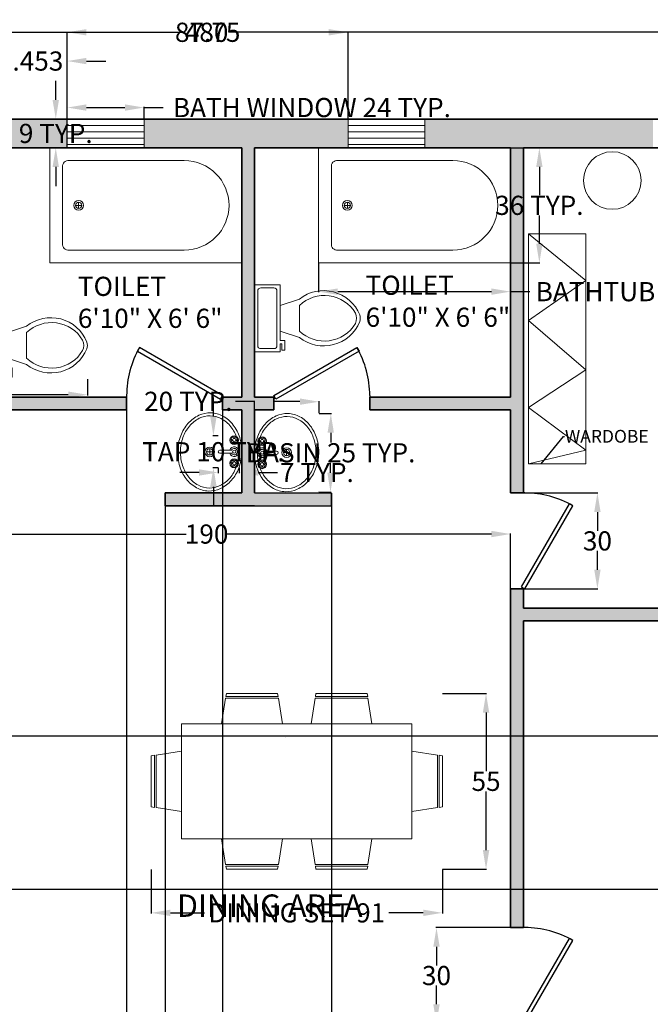
# Model space of a CAD drawing. Units: inches. Extents: x -16 to 578, y -553 to 49.
# Tile 4 of 5: x 205 to 402, y -259 to 49. Entities that reach past the tile are written whole.
import ezdxf
from ezdxf import colors
from ezdxf.entities.mleader import LeaderData, LeaderLine
from ezdxf.math import Vec2, Vec3

# ---------------------------------------------------------------- set-up
doc = ezdxf.new("R2010")
doc.units = ezdxf.units.IN
doc.header["$MEASUREMENT"] = 0
for name, color, linetype, lineweight in [('A-ANNO-DIMS', 2, 'Continuous', 18), ('A-ANNO-TEXT', 7, 'Continuous', 18), ('A-AREA-IDEN', 7, 'Continuous', 25), ('A-DOOR', 3, 'Continuous', 25), ('A-FLOR-CASE', 8, 'Continuous', 18), ('A-FLOR-FIXT', 9, 'Continuous', 18), ('A-FURN', 8, 'Continuous', 18), ('A-GLAZ', 4, 'Continuous', 18), ('A-WALL', 7, 'Continuous', 35)]:
    doc.layers.add(name, color=color, linetype=linetype, lineweight=lineweight)
doc.layers.add('A-WALL-PATT', color=251, linetype='Continuous', lineweight=13, true_color=0x636466)
doc.styles.get("Standard").update_dxf_attribs({"font": 'arial.ttf'})
doc.dimstyles.get("Standard").update_dxf_attribs({"dimtxt": 6, "dimasz": 6, "dimexe": 0.18, "dimexo": 0.0625, "dimgap": 0.09, "dimtad": 0, "dimtih": 1, "dimtoh": 1, "dimdec": 0, "dimzin": 0, "dimdsep": 46, "dimlunit": 4, "dimtxsty": 'Standard', "dimcen": 0.09, "dimadec": 0, "dimazin": 0, "dimtfac": 1, "dimtdec": 0, "dimtofl": 0, "dimtmove": 0, "dimatfit": 3, "dimfxl": 1, "dimtolj": 1, "dimtzin": 0, "dimarcsym": 0})

# ---------------------------------------------------------------- blocks, each defined once
blk = doc.blocks.new('*U4')
for p, q in [((0, 0), (0, -6)), ((-40, 0), (-40, -6))]:
    blk.add_line(p, q)
blk.add_lwpolyline([(0, 0), (-34.64, 20), (-35.52, 18.48), (-0.88, -1.52)], close=True)
blk.add_arc((0, 0), 40, 150, 180)
blk = doc.blocks.new('*U2')
for p, q in [((0, 0), (0, -6)), ((40, 0), (40, -6))]:
    blk.add_line(p, q)
blk.add_lwpolyline([(0, 0), (34.64, 20), (35.52, 18.48), (0.87, -1.52)], close=True)
blk.add_arc((0, 0), 40, 0, 30)
blk = doc.blocks.new('Toilet - top')
for p, q in [((9.5, -6), (9.5, -2)), ((-10, -8.5), (-8, -8.5)), ((-10, -9.5), (-10, -8.5)), ((-8, -8.5), (-8, -8)), ((-7, -8), (-7, -9.5)), ((-4, -8), (-6, -14)), ((4, -8), (6, -14)), ((-7, -9.5), (-10, -9.5)), ((4, -14), (-4, -14))]:
    blk.add_line(p, q)
for points in [[(-7, -8), (10.5, -8), (10.5, 0), (-10.5, 0), (-10.5, -8), (-8, -8)], [(-9.5, -2), (-9.5, -6)], [(8.5, -1), (-8.5, -1)], [(-8.5, -7), (8.5, -7)]]:
    blk.add_lwpolyline(points)
for centre, radius, start, end in [((-8.62, -1.88), 0.884, 81.8699, 188.1301), ((8.62, -1.88), 0.884, 351.8699, 98.1301), ((-8.62, -6.12), 0.884, 171.8699, 278.1301), ((8.62, -6.12), 0.884, 261.8699, 8.1301), ((3.52, -21.58), 12.17, 141.4691, 247.9714), ((4.2, -21.82), 11.33, 136.3677, 238.9468), ((-3.52, -21.58), 12.17, 292.0284, 38.5307), ((-4.2, -21.82), 11.33, 301.053, 43.6321), ((0, -27.88), 4, 245.7318, 294.2682), ((0, -29), 4, 254.8605, 285.1395)]:
    blk.add_arc(centre, radius, start, end)
blk = doc.blocks.new('Bath Tub - 26 x 60 in.')
for p, q in [((8, -18), (10, -18)), ((9, -17), (9, -19))]:
    blk.add_line(p, q)
blk.add_lwpolyline([(0, -36), (0, 0), (60, 0), (60, -36)], close=True)
for points in [[(4, -30), (4, -6)], [(6, -4), (42, -4)], [(42, -32), (6, -32)]]:
    blk.add_lwpolyline(points)
for radius in [1.5, 1]:
    blk.add_circle((9, -18), radius)
for centre, radius, start, end in [((5.75, -5.75), 1.77, 81.8699, 188.1301), ((42, -18), 14, 270, 90), ((5.75, -30.25), 1.77, 171.8699, 278.1301)]:
    blk.add_arc(centre, radius, start, end)
blk = doc.blocks.new('Sink - Oval top')
for p, q in [((-1, 0), (1, 0)), ((0, 1), (0, -1))]:
    blk.add_line(p, q)
for points in [[(-12.23, 0.39, 0.117634), (-11.46, -3.36, 0.104469), (-8.88, -6.8, 0.090016), (-5.08, -9.07, 0.08192), (-0.32, -10.02, 0.08192), (4.49, -9.38, 0.090016), (8.42, -7.36, 0.104469), (11.22, -4.09, 0.117634), (12.23, -0.39, 0.117634), (11.46, 3.36, 0.104469), (8.88, 6.8, 0.090016), (5.08, 9.07, 0.08192), (0.32, 10.02, 0.08192), (-4.49, 9.38, 0.090016), (-8.42, 7.36, 0.104469), (-11.22, 4.09, 0.117634)], [(-11.29, 0.16, 0.118622), (-10.52, -3.25, 0.104678), (-8.07, -6.36, 0.089562), (-4.54, -8.37, 0.081185), (-0.13, -9.15, 0.081185), (4.3, -8.49, 0.089562), (7.89, -6.58, 0.104678), (10.42, -3.55, 0.118622), (11.29, -0.16, 0.118622), (10.52, 3.25, 0.104678), (8.07, 6.36, 0.089562), (4.54, 8.37, 0.081185), (0.13, 9.15, 0.081185), (-4.3, 8.49, 0.089562), (-7.89, 6.58, 0.104678), (-10.42, 3.55, 0.118622)]]:
    blk.add_lwpolyline(points, format="xyb", close=True)
for radius in [1.5, 1]:
    blk.add_circle((0, 0), radius)
blk = doc.blocks.new('Faucet - Bathroom top')
for p, q in [((-4.107, 0.125), (-4.375, 0.125)), ((-3.75, 0.4788), (-3.75, 0.75)), ((-3.5, 0.482), (-3.5, 0.75)), ((-3.1461, 0.125), (-2.875, 0.125)), ((3.143, 0.125), (2.875, 0.125)), ((3.5, 0.4788), (3.5, 0.75)), ((3.75, 0.482), (3.75, 0.75)), ((4.1039, 0.125), (4.375, 0.125)), ((-4.1039, -0.125), (-4.375, -0.125)), ((-3.75, -0.4821), (-3.75, -0.75)), ((-3.5, -0.4789), (-3.5, -0.75)), ((-3.143, -0.125), (-2.875, -0.125)), ((-0.5, -0.8639), (-0.5, -4.5)), ((0.5, -4.5), (0.5, -0.8631)), ((3.1461, -0.125), (2.875, -0.125)), ((3.5, -0.4821), (3.5, -0.75)), ((3.75, -0.4789), (3.75, -0.75)), ((4.107, -0.125), (4.375, -0.125))]:
    blk.add_line(p, q)
for centre, radius in [((-3.625, 0), 1.375), ((-4.625, 0), 0.2795), ((-3.625, 0), 0.5), ((-3.625, 1), 0.2795), ((-2.625, 0), 0.2795), ((0, 0), 0.5), ((3.625, 0), 1.375), ((2.625, 0), 0.2795), ((3.625, 0), 0.5), ((3.625, 1), 0.2795), ((4.625, 0), 0.2795), ((-3.625, -1), 0.2795), ((3.625, -1), 0.2795)]:
    blk.add_circle(centre, radius)
for centre, radius, start, end in [((-3.625, 0), 1, 105.2407, 164.2093), ((-3.625, 0), 1, 16.44125, 74.07887), ((0, 0), 1.5, 289.6514, 250.3603), ((0, 0), 1, 300.3431, 239.7554), ((3.625, 0), 1, 106.12, 164.0884), ((3.625, 0), 1, 16.23422, 73.90469), ((-3.625, 0), 1, 196.2342, 253.9047), ((-3.625, 0), 1, 286.12, 344.0884), ((3.625, 0), 1, 196.4413, 254.0789), ((3.625, 0), 1, 285.2407, 344.2093), ((0, -4.5), 0.5, 180, 0)]:
    blk.add_arc(centre, radius, start, end)
blk = doc.blocks.new('Dining Set - 36 x 72 in.')
for p, q in [((-22.2343, 26.00059), (-23.4847, 17.99762)), ((-22.2304, 26), (-5.7608, 26)), ((-22, 27.5), (-22.1562, 26.50042)), ((-5.8416, 26.5), (-22.1534, 26.5)), ((-22, 27.5), (-6, 27.5)), ((-5.8437, 26.49966), (-6, 27.5)), ((-4.5152, 17.99762), (-5.7655, 25.99926)), ((5.7657, 26.00059), (4.5153, 17.99762)), ((5.7696, 26), (22.2392, 26)), ((6, 27.5), (5.8438, 26.50042)), ((22.1584, 26.5), (5.8466, 26.5)), ((6, 27.5), (22, 27.5)), ((22.1563, 26.49966), (22, 27.5)), ((23.4848, 17.99762), (22.2345, 25.99926)), ((36, 18), (-36, 18)), ((-36, 18), (-36, -18)), ((36, -18), (36, 18)), ((-44.0006, 8.23428), (-35.9976, 9.48474)), ((44.0006, 8.23428), (35.9976, 9.48474)), ((-45.5, 8), (-44.5004, 8.15617)), ((-45.5, 8), (-45.5, -8)), ((-44.5, -8.15843), (-44.5, 8.15338)), ((-44, 8.23041), (-44, -8.23915)), ((44, 8.23041), (44, -8.23915)), ((44.5, -8.15843), (44.5, 8.15338)), ((45.5, 8), (44.5005, 8.15617)), ((45.5, 8), (45.5, -8)), ((-44.4997, -8.15631), (-45.5, -8)), ((-35.9976, -9.48476), (-43.9993, -8.2345)), ((35.9976, -9.48476), (43.9993, -8.2345)), ((44.4997, -8.15631), (45.5, -8)), ((-36, -18), (36, -18)), ((-22.2343, -26.0006), (-23.4847, -17.99762)), ((-4.5152, -17.99762), (-5.7655, -25.99928)), ((5.7657, -26.0006), (4.5153, -17.99762)), ((23.4848, -17.99762), (22.2345, -25.99928)), ((-22.2304, -26), (-5.7608, -26)), ((-22, -27.5), (-22.1562, -26.50044)), ((-5.8416, -26.5), (-22.1534, -26.5)), ((-22, -27.5), (-6, -27.5)), ((-5.8437, -26.49967), (-6, -27.5)), ((5.7696, -26), (22.2392, -26)), ((6, -27.5), (5.8438, -26.50044)), ((22.1584, -26.5), (5.8466, -26.5)), ((6, -27.5), (22, -27.5)), ((22.1563, -26.49967), (22, -27.5))]:
    blk.add_line(p, q)
blk.add_lwpolyline([(-3.6035, 13.63021), (-3.6035, 13.63021)], close=True)
blk = doc.blocks.new('WIN-24X9')
for p, q in [((-24, -2), (0, -2)), ((-24, -4), (0, -4)), ((-24, -6), (0, -6)), ((-24, -8), (0, -8))]:
    blk.add_line(p, q)
blk.add_lwpolyline([(0, 0), (0, -9), (-24, -9), (-24, 0)], close=True)
blk = doc.blocks.new('WARDROBE-72X18')
for p, q in [((0, 0), (18, -14.58)), ((18, -14.58), (0, -27.16)), ((0, -27.16), (18, -42.59)), ((18, -42.59), (0, -54.31)), ((0, -54.31), (18, -67.75)), ((18, -67.75), (0, -72))]:
    blk.add_line(p, q)
blk.add_lwpolyline([(0, 0), (18, 0), (18, -72), (0, -72)], close=True)
blk = doc.blocks.new('NIGHTSTAND-ROUND-18')
blk.add_circle((0, 0), 9)
blk = doc.blocks.new('*D38')
at = {"layer": 'A-ANNO-DIMS', "color": 0, "lineweight": -2, "transparency": 16777216}
for p, q in [((192.91, -63.14), (192.91, -68.22)), ((225.96, -63.14), (225.96, -68.22)), ((192.91, -68.04), (186.91, -68.04)), ((219.96, -68.04), (198.91, -68.04))]:
    blk.add_line(p, q, dxfattribs=at)
at = {"layer": 'A-ANNO-DIMS', "color": 0, "transparency": 16777216}
for points in [[(198.91, -67.04), (198.91, -69.04), (192.91, -68.04)], [(219.96, -67.04), (219.96, -69.04), (225.96, -68.04)]]:
    blk.add_solid(points, dxfattribs=at)
at = {"layer": 'Defpoints', "color": 0, "transparency": 16777216}
for p in [(192.91, -63.08), (225.96, -63.08), (192.91, -68.04)]:
    blk.add_point(p, dxfattribs=at)
at = {"layer": 'A-ANNO-DIMS', "color": 0, "transparency": 16777216, "insert": (163.95, -68.04), "char_height": 6, "attachment_point": 5}
blk.add_mtext('\\A1;WC 33 TYP.', dxfattribs=at)
blk = doc.blocks.new('*D40')
at = {"layer": 'A-ANNO-DIMS', "color": 0, "lineweight": -2, "transparency": 16777216}
for p, q in [((298.19, -26.83), (298.19, -35.95)), ((358.19, -26.83), (358.19, -35.95)), ((304.19, -35.77), (352.19, -35.77)), ((358.19, -35.77), (364.19, -35.77))]:
    blk.add_line(p, q, dxfattribs=at)
at = {"layer": 'A-ANNO-DIMS', "color": 0, "transparency": 16777216}
for points in [[(304.19, -34.77), (304.19, -36.77), (298.19, -35.77)], [(352.19, -34.77), (352.19, -36.77), (358.19, -35.77)]]:
    blk.add_solid(points, dxfattribs=at)
at = {"layer": 'Defpoints', "color": 0, "transparency": 16777216}
for p in [(298.19, -26.77), (358.19, -26.77), (358.19, -35.77)]:
    blk.add_point(p, dxfattribs=at)
at = {"layer": 'A-ANNO-DIMS', "color": 0, "transparency": 16777216, "insert": (399.47, -35.77), "char_height": 6, "attachment_point": 5}
blk.add_mtext('\\A1;BATHTUB 60 TYP.', dxfattribs=at)
blk = doc.blocks.new('*D41')
at = {"layer": 'A-ANNO-DIMS', "color": 0, "lineweight": -2, "transparency": 16777216}
for p, q in [((358.25, 9.23), (367.37, 9.23)), ((367.19, 3.23), (367.19, -5.61)), ((367.19, -20.77), (367.19, -11.92)), ((358.25, -26.77), (367.37, -26.77))]:
    blk.add_line(p, q, dxfattribs=at)
at = {"layer": 'A-ANNO-DIMS', "color": 0, "transparency": 16777216}
for points in [[(366.19, 3.23), (368.19, 3.23), (367.19, 9.23)], [(366.19, -20.77), (368.19, -20.77), (367.19, -26.77)]]:
    blk.add_solid(points, dxfattribs=at)
at = {"layer": 'Defpoints', "color": 0, "transparency": 16777216}
for p in [(358.19, 9.23), (367.19, 9.23), (358.19, -26.77)]:
    blk.add_point(p, dxfattribs=at)
at = {"layer": 'A-ANNO-DIMS', "color": 0, "transparency": 16777216, "insert": (367.19, -8.77), "char_height": 6, "attachment_point": 5}
blk.add_mtext('\\A1;36 TYP.', dxfattribs=at)
blk = doc.blocks.new('*D44')
at = {"layer": 'A-ANNO-DIMS', "color": 0, "lineweight": -2, "transparency": 16777216}
for p, q in [((298.39, -73.9), (302.19, -73.92)), ((301.98, -79.92), (301.97, -83)), ((301.93, -92.47), (301.94, -89.38)), ((298.28, -98.45), (302.08, -98.47))]:
    blk.add_line(p, q, dxfattribs=at)
at = {"layer": 'A-ANNO-DIMS', "color": 0, "transparency": 16777216}
for points in [[(300.98, -79.91), (302.98, -79.92), (302.01, -73.92)], [(300.93, -92.46), (302.93, -92.47), (301.9, -98.47)]]:
    blk.add_solid(points, dxfattribs=at)
at = {"layer": 'Defpoints', "color": 0, "transparency": 16777216}
for p in [(298.32, -73.9), (302.01, -73.92), (298.22, -98.45)]:
    blk.add_point(p, dxfattribs=at)
at = {"layer": 'A-ANNO-DIMS', "color": 0, "transparency": 16777216, "insert": (301.95, -86.19), "char_height": 6, "attachment_point": 5}
blk.add_mtext('\\A1;BASIN 25 TYP.', dxfattribs=at)
blk = doc.blocks.new('*D45')
at = {"layer": 'A-ANNO-DIMS', "color": 0, "lineweight": -2, "transparency": 16777216}
for p, q in [((278.2, -70.13), (272.2, -70.1)), ((278.19, -73.75), (278.2, -69.95)), ((292.34, -70.19), (284.2, -70.16)), ((298.32, -73.84), (298.34, -70.04))]:
    blk.add_line(p, q, dxfattribs=at)
at = {"layer": 'A-ANNO-DIMS', "color": 0, "transparency": 16777216}
for points in [[(284.21, -69.16), (284.2, -71.16), (278.2, -70.13)], [(292.34, -69.19), (292.34, -71.19), (298.34, -70.22)]]:
    blk.add_solid(points, dxfattribs=at)
at = {"layer": 'Defpoints', "color": 0, "transparency": 16777216}
for p in [(278.2, -70.13), (278.19, -73.81), (298.32, -73.9)]:
    blk.add_point(p, dxfattribs=at)
at = {"layer": 'A-ANNO-DIMS', "color": 0, "transparency": 16777216, "insert": (257.46, -70.1), "char_height": 6, "attachment_point": 5}
blk.add_mtext('\\A1;20 TYP.', dxfattribs=at)
blk = doc.blocks.new('*D46')
at = {"layer": 'A-ANNO-DIMS', "color": 0, "lineweight": -2, "transparency": 16777216}
for p, q in [((265.32, -74.86), (265.32, -68.86)), ((266.75, -80.86), (265.14, -80.86)), ((266.75, -90.86), (265.14, -90.86)), ((265.32, -96.86), (265.32, -102.86))]:
    blk.add_line(p, q, dxfattribs=at)
at = {"layer": 'A-ANNO-DIMS', "color": 0, "transparency": 16777216}
for points in [[(264.32, -74.86), (266.32, -74.86), (265.32, -80.86)], [(264.32, -96.86), (266.32, -96.86), (265.32, -90.86)]]:
    blk.add_solid(points, dxfattribs=at)
at = {"layer": 'Defpoints', "color": 0, "transparency": 16777216}
for p in [(266.82, -80.86), (265.32, -90.86), (266.82, -90.86)]:
    blk.add_point(p, dxfattribs=at)
at = {"layer": 'A-ANNO-DIMS', "color": 0, "transparency": 16777216, "insert": (265.32, -85.86), "char_height": 6, "attachment_point": 5}
blk.add_mtext('\\A1;TAP 10 TYP.', dxfattribs=at)
blk = doc.blocks.new('*D47')
at = {"layer": 'A-ANNO-DIMS', "color": 0, "lineweight": -2, "transparency": 16777216}
for p, q in [((260.82, -92.36), (254.82, -92.36)), ((266.82, -90.92), (266.82, -92.54)), ((273.32, -90.92), (273.32, -92.54)), ((279.32, -92.36), (285.32, -92.36))]:
    blk.add_line(p, q, dxfattribs=at)
at = {"layer": 'A-ANNO-DIMS', "color": 0, "transparency": 16777216}
for points in [[(260.82, -91.36), (260.82, -93.36), (266.82, -92.36)], [(279.32, -91.36), (279.32, -93.36), (273.32, -92.36)]]:
    blk.add_solid(points, dxfattribs=at)
at = {"layer": 'Defpoints', "color": 0, "transparency": 16777216}
for p in [(266.82, -90.86), (273.32, -90.86), (273.32, -92.36)]:
    blk.add_point(p, dxfattribs=at)
at = {"layer": 'A-ANNO-DIMS', "color": 0, "transparency": 16777216, "insert": (297.66, -92.36), "char_height": 6, "attachment_point": 5}
blk.add_mtext('\\A1;7 TYP.', dxfattribs=at)
blk = doc.blocks.new('*D48')
at = {"layer": 'A-ANNO-DIMS', "color": 0, "lineweight": -2, "transparency": 16777216}
for p, q in [((219.64, 18.3), (219.64, 22.01)), ((225.64, 21.83), (237.64, 21.83)), ((243.64, 18.3), (243.64, 22.01)), ((243.64, 21.83), (249.64, 21.83))]:
    blk.add_line(p, q, dxfattribs=at)
at = {"layer": 'A-ANNO-DIMS', "color": 0, "transparency": 16777216}
for points in [[(225.64, 22.83), (225.64, 20.83), (219.64, 21.83)], [(237.64, 22.83), (237.64, 20.83), (243.64, 21.83)]]:
    blk.add_solid(points, dxfattribs=at)
at = {"layer": 'Defpoints', "color": 0, "transparency": 16777216}
for p in [(243.64, 21.83), (219.64, 18.23), (243.64, 18.23)]:
    blk.add_point(p, dxfattribs=at)
at = {"layer": 'A-ANNO-DIMS', "color": 0, "transparency": 16777216, "insert": (296.1, 21.83), "char_height": 6, "attachment_point": 5}
blk.add_mtext('\\A1;BATH WINDOW 24 TYP.', dxfattribs=at)
blk = doc.blocks.new('*D49')
at = {"layer": 'A-ANNO-DIMS', "color": 0, "lineweight": -2, "transparency": 16777216}
for p, q in [((216.04, 24.23), (216.04, 30.23)), ((219.58, 18.23), (215.86, 18.23)), ((219.58, 9.23), (215.86, 9.23)), ((216.04, 3.23), (216.04, -2.77))]:
    blk.add_line(p, q, dxfattribs=at)
at = {"layer": 'A-ANNO-DIMS', "color": 0, "transparency": 16777216}
for points in [[(215.04, 24.23), (217.04, 24.23), (216.04, 18.23)], [(215.04, 3.23), (217.04, 3.23), (216.04, 9.23)]]:
    blk.add_solid(points, dxfattribs=at)
at = {"layer": 'Defpoints', "color": 0, "transparency": 16777216}
for p in [(216.04, 18.23), (219.64, 18.23), (219.64, 9.23)]:
    blk.add_point(p, dxfattribs=at)
at = {"layer": 'A-ANNO-DIMS', "color": 0, "transparency": 16777216, "insert": (216.04, 13.73), "char_height": 6, "attachment_point": 5}
blk.add_mtext('\\A1;9 TYP.', dxfattribs=at)
blk = doc.blocks.new('*D60')
at = {"layer": 'A-ANNO-DIMS', "color": 0, "lineweight": -2, "transparency": 16777216}
for p, q in [((245.88, -216.56), (245.88, -230.33)), ((336.88, -216.56), (336.88, -230.33)), ((251.88, -230.15), (262.57, -230.15)), ((330.88, -230.15), (320.18, -230.15))]:
    blk.add_line(p, q, dxfattribs=at)
at = {"layer": 'A-ANNO-DIMS', "color": 0, "transparency": 16777216}
for points in [[(251.88, -229.15), (251.88, -231.15), (245.88, -230.15)], [(330.88, -229.15), (330.88, -231.15), (336.88, -230.15)]]:
    blk.add_solid(points, dxfattribs=at)
at = {"layer": 'Defpoints', "color": 0, "transparency": 16777216}
for p in [(245.88, -216.5), (336.88, -216.5), (336.88, -230.15)]:
    blk.add_point(p, dxfattribs=at)
at = {"layer": 'A-ANNO-DIMS', "color": 0, "transparency": 16777216, "insert": (291.38, -230.15), "char_height": 6, "attachment_point": 5}
blk.add_mtext('\\A1;DINING SET 91', dxfattribs=at)
blk = doc.blocks.new('*D61')
at = {"layer": 'A-ANNO-DIMS', "color": 0, "lineweight": -2, "transparency": 16777216}
for p, q in [((336.94, -161.5), (350.71, -161.5)), ((350.53, -167.5), (350.53, -185.86)), ((350.53, -210.5), (350.53, -192.14)), ((336.94, -216.5), (350.71, -216.5))]:
    blk.add_line(p, q, dxfattribs=at)
at = {"layer": 'A-ANNO-DIMS', "color": 0, "transparency": 16777216}
for points in [[(349.53, -167.5), (351.53, -167.5), (350.53, -161.5)], [(349.53, -210.5), (351.53, -210.5), (350.53, -216.5)]]:
    blk.add_solid(points, dxfattribs=at)
at = {"layer": 'Defpoints', "color": 0, "transparency": 16777216}
for p in [(336.88, -161.5), (350.53, -161.5), (336.88, -216.5)]:
    blk.add_point(p, dxfattribs=at)
at = {"layer": 'A-ANNO-DIMS', "color": 0, "transparency": 16777216, "insert": (350.53, -189), "char_height": 6, "attachment_point": 5}
blk.add_mtext('\\A1;55', dxfattribs=at)
blk = doc.blocks.new('*D62')
at = {"layer": 'A-ANNO-DIMS', "color": 0, "lineweight": -2, "transparency": 16777216}
for p, q in [((23.19, 18.3), (23.19, 45.56)), ((29.19, 45.38), (256.36, 45.38)), ((497.19, 45.38), (270.02, 45.38)), ((503.19, 18.3), (503.19, 45.56))]:
    blk.add_line(p, q, dxfattribs=at)
at = {"layer": 'A-ANNO-DIMS', "color": 0, "transparency": 16777216}
for points in [[(29.19, 46.38), (29.19, 44.38), (23.19, 45.38)], [(497.19, 46.38), (497.19, 44.38), (503.19, 45.38)]]:
    blk.add_solid(points, dxfattribs=at)
at = {"layer": 'Defpoints', "color": 0, "transparency": 16777216}
for p in [(503.19, 45.38), (23.19, 18.23), (503.19, 18.23)]:
    blk.add_point(p, dxfattribs=at)
at = {"layer": 'A-ANNO-DIMS', "color": 0, "transparency": 16777216, "insert": (263.19, 45.38), "char_height": 6, "attachment_point": 5}
blk.add_mtext('\\A1;480', dxfattribs=at)
blk = doc.blocks.new('*D69')
at = {"layer": 'A-ANNO-DIMS', "color": 0, "lineweight": -2, "transparency": 16777216}
for p, q in [((168.25, -174.77), (530.52, -174.77)), ((530.34, -180.77), (530.34, -195.61)), ((530.34, -216.77), (530.34, -201.92)), ((168.25, -222.77), (530.52, -222.77))]:
    blk.add_line(p, q, dxfattribs=at)
at = {"layer": 'A-ANNO-DIMS', "color": 0, "transparency": 16777216}
for points in [[(529.34, -180.77), (531.34, -180.77), (530.34, -174.77)], [(529.34, -216.77), (531.34, -216.77), (530.34, -222.77)]]:
    blk.add_solid(points, dxfattribs=at)
at = {"layer": 'Defpoints', "color": 0, "transparency": 16777216}
for p in [(168.19, -174.77), (168.19, -222.77), (530.34, -222.77)]:
    blk.add_point(p, dxfattribs=at)
at = {"layer": 'A-ANNO-DIMS', "color": 0, "transparency": 16777216, "insert": (530.34, -198.77), "char_height": 6, "attachment_point": 5}
blk.add_mtext('\\A1;48', dxfattribs=at)
blk = doc.blocks.new('*D70')
at = {"layer": 'A-ANNO-DIMS', "color": 0, "lineweight": -2, "transparency": 16777216}
for p, q in [((362.13, -234.77), (334.86, -234.77)), ((335.04, -240.77), (335.04, -246.61)), ((335.04, -258.77), (335.04, -252.92)), ((362.13, -264.77), (334.86, -264.77))]:
    blk.add_line(p, q, dxfattribs=at)
at = {"layer": 'A-ANNO-DIMS', "color": 0, "transparency": 16777216}
for points in [[(334.04, -240.77), (336.04, -240.77), (335.04, -234.77)], [(334.04, -258.77), (336.04, -258.77), (335.04, -264.77)]]:
    blk.add_solid(points, dxfattribs=at)
at = {"layer": 'Defpoints', "color": 0, "transparency": 16777216}
for p in [(335.04, -234.77), (362.19, -234.77), (362.19, -264.77)]:
    blk.add_point(p, dxfattribs=at)
at = {"layer": 'A-ANNO-DIMS', "color": 0, "transparency": 16777216, "insert": (335.04, -249.77), "char_height": 6, "attachment_point": 5}
blk.add_mtext('\\A1;30', dxfattribs=at)
blk = doc.blocks.new('*D72')
at = {"layer": 'A-ANNO-DIMS', "color": 0, "lineweight": -2, "transparency": 16777216}
for p, q in [((186.19, 36.38), (180.19, 36.38)), ((192.19, 9.3), (192.19, 36.56)), ((219.64, 9.3), (219.64, 36.56)), ((225.64, 36.38), (231.64, 36.38))]:
    blk.add_line(p, q, dxfattribs=at)
at = {"layer": 'A-ANNO-DIMS', "color": 0, "transparency": 16777216}
for points in [[(186.19, 37.38), (186.19, 35.38), (192.19, 36.38)], [(225.64, 37.38), (225.64, 35.38), (219.64, 36.38)]]:
    blk.add_solid(points, dxfattribs=at)
at = {"layer": 'Defpoints', "color": 0, "transparency": 16777216}
for p in [(219.64, 36.38), (192.19, 9.23), (219.64, 9.23)]:
    blk.add_point(p, dxfattribs=at)
at = {"layer": 'A-ANNO-DIMS', "color": 0, "transparency": 16777216, "insert": (205.91, 36.38), "char_height": 6, "attachment_point": 5}
blk.add_mtext('\\A1;27.453', dxfattribs=at)
blk = doc.blocks.new('*D73')
at = {"layer": 'A-ANNO-DIMS', "color": 0, "lineweight": -2, "transparency": 16777216}
for p, q in [((219.64, 18.3), (219.64, 45.56)), ((225.64, 45.38), (253.28, 45.38)), ((301.39, 45.38), (273.76, 45.38)), ((307.39, 18.3), (307.39, 45.56))]:
    blk.add_line(p, q, dxfattribs=at)
at = {"layer": 'A-ANNO-DIMS', "color": 0, "transparency": 16777216}
for points in [[(225.64, 46.38), (225.64, 44.38), (219.64, 45.38)], [(301.39, 46.38), (301.39, 44.38), (307.39, 45.38)]]:
    blk.add_solid(points, dxfattribs=at)
at = {"layer": 'Defpoints', "color": 0, "transparency": 16777216}
for p in [(307.39, 45.38), (219.64, 18.23), (307.39, 18.23)]:
    blk.add_point(p, dxfattribs=at)
at = {"layer": 'A-ANNO-DIMS', "color": 0, "transparency": 16777216, "insert": (263.52, 45.38), "char_height": 6, "attachment_point": 5}
blk.add_mtext('\\A1;87.75', dxfattribs=at)
blk = doc.blocks.new('*D81')
at = {"layer": 'A-ANNO-DIMS', "color": 0, "lineweight": -2, "transparency": 16777216}
for p, q in [((238.19, -72.83), (238.19, -549.1)), ((268.19, -72.83), (268.19, -549.1)), ((244.19, -548.92), (248.81, -548.92)), ((262.19, -548.92), (257.56, -548.92))]:
    blk.add_line(p, q, dxfattribs=at)
at = {"layer": 'A-ANNO-DIMS', "color": 0, "transparency": 16777216}
for points in [[(244.19, -547.92), (244.19, -549.92), (238.19, -548.92)], [(262.19, -547.92), (262.19, -549.92), (268.19, -548.92)]]:
    blk.add_solid(points, dxfattribs=at)
at = {"layer": 'Defpoints', "color": 0, "transparency": 16777216}
for p in [(238.19, -72.77), (268.19, -72.77), (268.19, -548.92)]:
    blk.add_point(p, dxfattribs=at)
at = {"layer": 'A-ANNO-DIMS', "color": 0, "transparency": 16777216, "insert": (253.19, -548.92), "char_height": 6, "attachment_point": 5}
blk.add_mtext('\\A1;30', dxfattribs=at)
blk = doc.blocks.new('*D82')
at = {"layer": 'A-ANNO-DIMS', "color": 0, "lineweight": -2, "transparency": 16777216}
for p, q in [((250.19, -102.83), (250.19, -549.1)), ((302.19, -102.91), (302.19, -549.1)), ((256.19, -548.92), (271.83, -548.92)), ((296.19, -548.92), (280.54, -548.92))]:
    blk.add_line(p, q, dxfattribs=at)
at = {"layer": 'A-ANNO-DIMS', "color": 0, "transparency": 16777216}
for points in [[(256.19, -547.92), (256.19, -549.92), (250.19, -548.92)], [(296.19, -547.92), (296.19, -549.92), (302.19, -548.92)]]:
    blk.add_solid(points, dxfattribs=at)
at = {"layer": 'Defpoints', "color": 0, "transparency": 16777216}
for p in [(250.19, -102.77), (302.19, -102.85), (302.19, -548.92)]:
    blk.add_point(p, dxfattribs=at)
at = {"layer": 'A-ANNO-DIMS', "color": 0, "transparency": 16777216, "insert": (276.19, -548.92), "char_height": 6, "attachment_point": 5}
blk.add_mtext('\\A1;52', dxfattribs=at)
blk = doc.blocks.new('*D83')
at = {"layer": 'A-ANNO-DIMS', "color": 0, "lineweight": -2, "transparency": 16777216}
for p, q in [((168.19, -138.7), (168.19, -111.44)), ((174.19, -111.62), (256.76, -111.62)), ((352.19, -111.62), (269.61, -111.62)), ((358.19, -138.7), (358.19, -111.44))]:
    blk.add_line(p, q, dxfattribs=at)
at = {"layer": 'A-ANNO-DIMS', "color": 0, "transparency": 16777216}
for points in [[(174.19, -110.62), (174.19, -112.62), (168.19, -111.62)], [(352.19, -110.62), (352.19, -112.62), (358.19, -111.62)]]:
    blk.add_solid(points, dxfattribs=at)
at = {"layer": 'Defpoints', "color": 0, "transparency": 16777216}
for p in [(358.19, -111.62), (168.19, -138.77), (358.19, -138.77)]:
    blk.add_point(p, dxfattribs=at)
at = {"layer": 'A-ANNO-DIMS', "color": 0, "transparency": 16777216, "insert": (263.19, -111.62), "char_height": 6, "attachment_point": 5}
blk.add_mtext('\\A1;190', dxfattribs=at)
blk = doc.blocks.new('*D84')
at = {"layer": 'A-ANNO-DIMS', "color": 0, "lineweight": -2, "transparency": 16777216}
for p, q in [((358.25, -98.77), (385.52, -98.77)), ((385.34, -104.77), (385.34, -110.61)), ((385.34, -122.77), (385.34, -116.92)), ((358.25, -128.77), (385.52, -128.77))]:
    blk.add_line(p, q, dxfattribs=at)
at = {"layer": 'A-ANNO-DIMS', "color": 0, "transparency": 16777216}
for points in [[(384.34, -104.77), (386.34, -104.77), (385.34, -98.77)], [(384.34, -122.77), (386.34, -122.77), (385.34, -128.77)]]:
    blk.add_solid(points, dxfattribs=at)
at = {"layer": 'Defpoints', "color": 0, "transparency": 16777216}
for p in [(358.19, -98.77), (358.19, -128.77), (385.34, -128.77)]:
    blk.add_point(p, dxfattribs=at)
at = {"layer": 'A-ANNO-DIMS', "color": 0, "transparency": 16777216, "insert": (385.34, -113.77), "char_height": 6, "attachment_point": 5}
blk.add_mtext('\\A1;30', dxfattribs=at)

msp = doc.modelspace()

# ---------------------------------------------------------------- hatches: boundary and pattern name
at = {"layer": 'A-WALL-PATT'}
h = msp.add_hatch(color=256, dxfattribs=at)
h.dxf.hatch_style = 1
h.paths.add_polyline_path([(32.1882, 9.2337), (89.8211, 9.2337), (89.8211, 18.2337), (23.1882, 18.2337), (23.1882, -55.5259), (32.1882, -55.5259)])
h.paths.add_polyline_path([(219.6411, 18.2337), (137.8211, 18.2337), (137.8211, 9.2337), (146.4179, 9.2337), (188.1882, 9.2337), (188.1882, -98.7663), (192.1882, -98.7663), (192.1882, -72.7663), (238.1882, -72.7663), (238.1882, -68.7663), (192.1882, -68.7663), (192.1882, 9.2337), (219.6411, 9.2337)])
h.paths.add_polyline_path([(307.3924, 18.2337), (243.6411, 18.2337), (243.6411, 9.2337), (274.1882, 9.2337), (274.1882, -26.7663), (274.1882, -68.7663), (268.1882, -68.7663), (268.1882, -72.7663), (274.1882, -72.7663), (274.1882, -98.7663), (250.1882, -98.7663), (250.1882, -102.7663), (274.1882, -102.7663), (278.1882, -102.7663), (302.188, -102.8481), (302.188, -98.8481), (278.1882, -98.7663), (278.1882, -86.8559, -0.01827889), (278.1882, -85.7663), (278.1882, -72.7663), (284.1882, -72.7663), (284.1882, -68.7663), (278.1882, -68.7663), (278.1882, 9.2337), (307.3924, 9.2337)])
h.paths.add_polyline_path([(402.6701, 18.2337), (331.3924, 18.2337), (331.3924, 9.2337), (358.1882, 9.2337), (358.1882, -26.7663), (358.1882, -68.7663), (314.1882, -68.7663), (314.1882, -72.7663), (358.1882, -72.7663), (358.1882, -98.7663), (362.1882, -98.7663), (362.1882, 9.2337), (402.6701, 9.2337)])
h.paths.add_polyline_path([(503.1882, 18.2337), (450.6701, 18.2337), (450.6701, 9.2337), (462.8072, 9.2337), (494.1882, 9.2337), (494.1882, -38.053), (503.1882, -38.053)])
h.paths.add_polyline_path([(503.1882, -86.053), (494.1882, -86.053), (494.1882, -134.7663), (362.1882, -134.7663), (362.1882, -128.7663), (358.1882, -128.7663), (358.1882, -138.7663), (358.1882, -234.7663), (362.1882, -234.7663), (362.1882, -138.7663), (494.1882, -138.7663), (494.1882, -181.1501), (503.1882, -181.1501)])
h.paths.add_polyline_path([(503.1882, -229.1501), (494.1882, -229.1501), (494.1882, -270.7663), (362.1882, -270.7663), (362.1882, -264.7663), (358.1882, -264.7663), (358.1882, -294.7663), (358.1882, -323.1753), (362.1882, -323.1753), (362.1882, -298.7663), (362.1882, -294.7663), (362.1882, -274.7663), (494.1882, -274.7663), (494.1882, -294.7663), (494.1882, -298.7663), (494.1882, -310.411), (503.1882, -310.411)])
h.paths.add_polyline_path([(503.1882, -358.411), (494.1882, -358.411), (494.1882, -394.7663), (362.1882, -394.7663), (362.1882, -353.1753), (358.1882, -353.1753), (358.1882, -398.7663), (494.1882, -398.7663), (494.1882, -512.7663), (451.8049, -512.7663), (451.8049, -521.7663), (503.1882, -521.7663)])
h.paths.add_polyline_path([(403.8049, -512.7663), (176.1882, -512.7663), (176.1882, -441.7663), (172.1882, -441.7663), (172.1882, -512.7663), (150.1882, -512.7663), (150.1882, -521.7663), (403.8049, -521.7663)])
h.paths.add_polyline_path([(176.1882, -258.7663), (168.1882, -258.7663), (168.1882, -246.7663), (168.1882, -234.7663), (168.1882, -222.7663), (164.1882, -222.7663), (164.1882, -234.7663), (164.1882, -258.7663), (102.0641, -258.7663), (102.0641, -262.7663), (168.1882, -262.7663), (172.1882, -262.7663), (172.1882, -333.7663), (176.1882, -333.7663), (176.1882, -262.7663)])
h.paths.add_polyline_path([(32.1882, -262.7663), (54.0641, -262.7663), (54.0641, -258.7663), (32.1882, -258.7663), (32.1882, -229.1501), (23.1882, -229.1501), (23.1882, -283.4909), (23.1882, -470.2771), (32.1882, -470.2771), (32.1882, -283.4909)])
h.paths.add_polyline_path([(32.1882, -103.5259), (23.1882, -103.5259), (23.1882, -181.1501), (32.1882, -181.1501)])
h.paths.add_polyline_path([(192.1882, -128.7663), (188.1882, -128.7663), (188.1882, -134.7663), (32.1882, -134.7663), (32.1882, -138.7663), (164.1882, -138.7663), (164.1882, -162.7663), (164.1882, -174.7663), (168.1882, -174.7663), (168.1882, -162.7663), (168.1882, -138.7663), (192.1882, -138.7663)])

# ---------------------------------------------------------------- linework, layer by layer
at = {"layer": 'A-WALL'}
for p, q in [((192.1882, 9.2337), (274.1882, 9.2337)), ((274.1882, -68.7663), (274.1882, 9.2337)), ((278.1882, 9.2337), (358.1882, 9.2337)), ((278.1882, -68.7663), (278.1882, 9.2337)), ((358.1882, 9.2337), (358.1882, -68.7663)), ((362.1882, 9.2337), (362.1882, -98.7663)), ((362.1882, 9.2337), (494.1882, 9.2337)), ((192.1882, -68.7663), (238.1882, -68.7663)), ((238.1882, -68.7663), (238.1882, -72.7663)), ((268.1882, -68.7663), (268.1882, -72.7663)), ((268.1882, -68.7663), (274.1882, -68.7663)), ((278.1882, -68.7663), (284.1882, -68.7663)), ((284.1882, -68.7663), (284.1882, -72.7663)), ((314.1882, -68.7663), (314.1882, -72.7663)), ((314.1882, -68.7663), (358.1882, -68.7663)), ((192.1882, -72.7663), (238.1882, -72.7663)), ((268.1882, -72.7663), (274.1882, -72.7663)), ((274.1882, -98.7663), (274.1882, -72.7663)), ((278.1882, -98.7663), (278.1882, -72.7663)), ((278.1882, -72.7663), (284.1882, -72.7663)), ((314.1882, -72.7663), (358.1882, -72.7663)), ((358.1882, -72.7663), (358.1882, -98.7663)), ((250.1882, -102.7663), (250.1882, -98.7663)), ((250.1882, -98.7663), (274.1882, -98.7663)), ((302.188, -98.8481), (278.1882, -98.7663)), ((302.188, -102.8481), (302.188, -98.8481)), ((358.1882, -98.7663), (362.1882, -98.7663)), ((274.1882, -102.7663), (250.1882, -102.7663)), ((274.1882, -102.7663), (278.1882, -102.7663)), ((278.1882, -102.7663), (302.188, -102.8481)), ((358.1882, -128.7663), (362.1882, -128.7663)), ((358.1882, -128.7663), (358.1882, -138.7663)), ((362.1882, -128.7663), (362.1882, -134.7663)), ((358.1882, -134.7663), (358.1882, -234.7663)), ((362.1882, -134.7663), (494.1882, -134.7663)), ((362.1882, -138.7663), (494.1882, -138.7663)), ((362.1882, -138.7663), (362.1882, -234.7663)), ((362.1882, -234.7663), (358.1882, -234.7663))]:
    msp.add_line(p, q, dxfattribs=at)
msp.add_lwpolyline([(23.1882, -283.4909), (23.1882, 18.2337), (503.1882, 18.2337), (503.1882, -521.7663), (150.1882, -521.7663)], dxfattribs=at)

# ---------------------------------------------------------------- block references
at = {"layer": 'A-DOOR', "xscale": 0.75, "yscale": 0.75, "zscale": 0.75}
for name, p in [('*U4', (268.1882, -68.2663)), ('*U2', (284.1882, -68.2663))]:
    msp.add_blockref(name, p, dxfattribs=at)
at = {"layer": 'A-DOOR', "xscale": 0.75, "yscale": 0.75, "zscale": 0.75, "rotation": 270}
for p in [(362.6882, -128.7663), (362.6882, -264.7663)]:
    msp.add_blockref('*U4', p, dxfattribs=at)
at = {"layer": 'A-FLOR-CASE'}
msp.add_blockref('WARDROBE-72X18', (363.7628, -17.6691), dxfattribs=at)
at = {"layer": 'A-FLOR-FIXT'}
for p in [(214.1882, 9.2337), (298.1882, 9.2337)]:
    msp.add_blockref('Bath Tub - 26 x 60 in.', p, dxfattribs=at)
for name, p, rotation in [('Toilet - top', (278.1882, -44.1107), 90), ('Toilet - top', (192.9126, -52.58), 90), ('Sink - Oval top', (264.1646, -85.9237), 270), ('Sink - Oval top', (288.2025, -86.1325), 89.7511563564458), ('Faucet - Bathroom top', (271.8175, -85.857), 270), ('Faucet - Bathroom top', (280.5494, -86.1659), 89.7511563564458)]:
    msp.add_blockref(name, p, dxfattribs=dict(at, rotation=rotation))
at = {"layer": 'A-FURN'}
for name, p in [('NIGHTSTAND-ROUND-18', (389.9693, -0.9972)), ('Dining Set - 36 x 72 in.', (291.3754, -188.9973))]:
    msp.add_blockref(name, p, dxfattribs=at)
at = {"layer": 'A-GLAZ'}
for p in [(243.6411, 18.2337), (331.3924, 18.2337)]:
    msp.add_blockref('WIN-24X9', p, dxfattribs=at)

# ---------------------------------------------------------------- texts
at = {"layer": 'A-AREA-IDEN', "attachment_point": 1}
for s, width, insert, char_height in [('TOILET\\P6\'10" X 6\' 6"', 55.766807, (312.8817, -30.7662), 6), ('TOILET\\P6\'10" X 6\' 6"', 55.766807, (222.9472, -31.1133), 6), ('DINING AREA', 91.835922, (253.9186, -224.3983), 7)]:
    msp.add_mtext_dynamic_manual_height_columns(s, width=width, gutter_width=1, heights=[0], dxfattribs=dict(at, insert=insert, char_height=char_height))

# ---------------------------------------------------------------- dimensions: what is measured, and where the dimension line sits
at = {"layer": 'A-ANNO-DIMS'}
for base, p1, p2, override, picture, middle in [((503.1882, 45.3837), (23.1882, 18.2337), (503.1882, 18.2337), {"dimdec": 0, "dimlfac": 1, "dimrnd": 0, "dimzin": 0, "dimdsep": 46, "dimlunit": 2}, '*D62', (263.1882, 45.3837)), ((307.3924, 45.3837), (219.6411, 18.2337), (307.3924, 18.2337), {"dimdec": 2, "dimlfac": 1, "dimrnd": 0, "dimzin": 0, "dimdsep": 46, "dimlunit": 2}, '*D73', (263.5168, 45.3837)), ((268.1882, -548.9163), (238.1882, -72.7663), (268.1882, -72.7663), {"dimdec": 0, "dimlfac": 1, "dimrnd": 0, "dimzin": 0, "dimdsep": 46, "dimlunit": 2}, '*D81', (253.1882, -548.9163)), ((302.188, -548.9163), (250.1882, -102.7663), (302.188, -102.8481), {"dimdec": 0, "dimlfac": 1, "dimrnd": 0, "dimzin": 0, "dimdsep": 46, "dimlunit": 2}, '*D82', (276.1881, -548.9163)), ((358.1882, -111.6163), (168.1882, -138.7663), (358.1882, -138.7663), {"dimdec": 0, "dimlfac": 1, "dimrnd": 0, "dimzin": 0, "dimdsep": 46, "dimlunit": 2}, '*D83', (263.1882, -111.6163))]:
    dim = msp.add_linear_dim(base=base, p1=p1, p2=p2, dimstyle='Standard', override=override, dxfattribs=at)
    dim.commit()
    dim.dimension.update_dxf_attribs({"geometry": picture, "text_midpoint": middle})
for base, p1, p2, angle, override, picture, middle in [((219.6411, 36.3837), (192.1882, 9.2337), (219.6411, 9.2337), 0, {"dimdec": 3, "dimlfac": 1, "dimrnd": 0, "dimzin": 0, "dimdsep": 46, "dimlunit": 2}, '*D72', (205.9146, 36.3837)), ((385.3382, -128.7663), (358.1882, -98.7663), (358.1882, -128.7663), 270, {"dimdec": 0, "dimlfac": 1, "dimrnd": 0, "dimzin": 0, "dimdsep": 46, "dimlunit": 2}, '*D84', (385.3382, -113.7663)), ((350.5254, -161.4973), (336.8754, -216.4973), (336.8754, -161.4973), 90, {"dimdec": 0, "dimlfac": 1, "dimrnd": 0, "dimzin": 0, "dimdsep": 46, "dimlunit": 2}, '*D61', (350.5254, -188.9973)), ((530.3382, -222.7663), (168.1882, -174.7663), (168.1882, -222.7663), 90, {"dimdec": 0, "dimlfac": 1, "dimrnd": 0, "dimzin": 0, "dimdsep": 46, "dimlunit": 2}, '*D69', (530.3382, -198.7663)), ((335.0382, -234.7663), (362.1882, -264.7663), (362.1882, -234.7663), 90, {"dimdec": 0, "dimlfac": 1, "dimrnd": 0, "dimzin": 0, "dimdsep": 46, "dimlunit": 2}, '*D70', (335.0382, -249.7663))]:
    dim = msp.add_linear_dim(base=base, p1=p1, p2=p2, angle=angle, dimstyle='Standard', override=override, dxfattribs=at)
    dim.commit()
    dim.dimension.update_dxf_attribs({"geometry": picture, "text_midpoint": middle})
for base, p1, p2, text, picture, middle in [((243.6411, 21.8337), (219.6411, 18.2337), (243.6411, 18.2337), 'BATH WINDOW <> TYP.', '*D48', (296.0961, 21.8337)), ((358.1882, -35.7663), (298.1882, -26.7663), (358.1882, -26.7663), 'BATHTUB <> TYP.', '*D40', (399.4719, -35.7663)), ((273.31753, -92.35703), (266.81745, -90.85703), (273.31753, -90.85703), '<> TYP.', '*D47', (297.65514, -92.35703)), ((336.8754, -230.1473), (245.8754, -216.4973), (336.8754, -216.4973), 'DINING SET <>', '*D60', (291.3754, -230.1473))]:
    dim = msp.add_linear_dim(base=base, p1=p1, p2=p2, text=text, dimstyle='Standard', override={"dimdec": 0, "dimlfac": 1, "dimrnd": 0, "dimzin": 0, "dimdsep": 46, "dimlunit": 2}, dxfattribs=at)
    dim.commit()
    dim.dimension.update_dxf_attribs({"geometry": picture, "text_midpoint": middle})
for base, p1, p2, angle, text, picture, middle in [((216.0411, 18.2337), (219.6411, 9.2337), (219.6411, 18.2337), 90, '<> TYP.', '*D49', (216.0411, 13.7337)), ((367.1882, 9.2337), (358.1882, -26.7663), (358.1882, 9.2337), 90, '<> TYP.', '*D41', (367.1882, -8.7663)), ((192.9126, -68.037), (225.9588, -63.08), (192.9126, -63.08), 180, 'WC <> TYP.', '*D38', (163.9501, -68.037)), ((278.2036, -70.1308), (298.324, -73.9009), (278.1876, -73.8134), 179.751156, '<> TYP.', '*D45', (257.4595, -70.1048)), ((265.3175, -90.857), (266.8175, -80.857), (266.8175, -90.857), 270, 'TAP <> TYP.', '*D46', (265.3175, -85.857)), ((302.0066, -73.9169), (298.2174, -98.4515), (298.324, -73.9009), 89.751156, 'BASIN <> TYP.', '*D44', (301.9533, -86.1922))]:
    dim = msp.add_linear_dim(base=base, p1=p1, p2=p2, angle=angle, text=text, dimstyle='Standard', override={"dimdec": 0, "dimlfac": 1, "dimrnd": 0, "dimzin": 0, "dimdsep": 46, "dimlunit": 2}, dxfattribs=at)
    dim.commit()
    dim.dimension.update_dxf_attribs({"geometry": picture, "text_midpoint": middle})

# ---------------------------------------------------------------- leaders
at = {"layer": 'A-ANNO-TEXT'}
ml = msp.add_multileader_mtext('Standard', dxfattribs=at)
ml.set_content('WARDOBE', color=256)
ml.set_leader_properties()
ml.build(insert=Vec2(0, 0))
ml.multileader.update_dxf_attribs({"dogleg_length": 0.36, "arrow_head_size": 0})
ctx = ml.context
ctx.base_point, ctx.arrow_head_size, ctx.landing_gap_size, ctx.plane_origin = Vec3(375.094, -81.0618), 0, 0.09, Vec3(367.7628, -89.6691)
notes = []
notes.append((ctx, [(0, (1, 1, 0), (374.734, -81.0618), (1, 0), 0.36, [(0, [(367.7628, -89.6691)], 0, [])])]))
ctx.mtext.insert, ctx.mtext.width, ctx.mtext.flow_direction = Vec3(375.184, -79.0277), 4, 5
for ctx, leaders in notes:
    for number, flags, end, landing, length, lines in leaders:
        leader = LeaderData()
        leader.index, (leader.has_last_leader_line, leader.has_dogleg_vector, leader.attachment_direction) = number, flags
        leader.last_leader_point, leader.dogleg_vector, leader.dogleg_length = Vec3(end), Vec3(landing), length
        for number, points, colour, breaks in lines:
            line = LeaderLine()
            line.index, line.vertices, line.color, line.breaks = number, Vec3.list(points), colors.encode_raw_color(colour), breaks
            leader.lines.append(line)
        ctx.leaders.append(leader)

doc.saveas('drawing.dxf')
